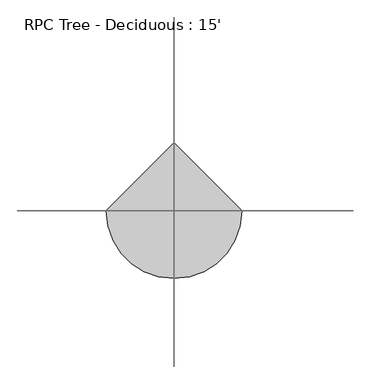
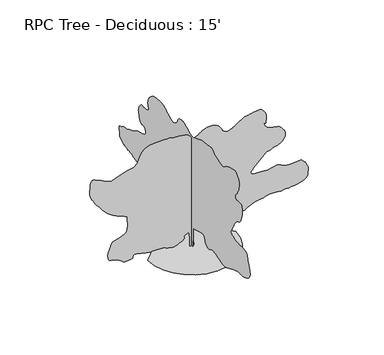
"""IFC4 building model written with IfcOpenShell, lengths in millimetres: geographic element geometry, RPC Tree - Deciduous : 15'."""

from ifc_helpers import new_model, si_unit, origin, place, context, project, spatial, triangles, source, transform, mapped, element, save


def rpc_tree_deciduous_15_10e6bd9b(model_context):
    return source(origin(), model_context, "Body", "Tessellation", [
        triangles([(0.0815727, 123.3442517, 0.0086663), (0.0815727, -127.150442, 0.0086663), (0.0815727, -142.8050915, 829.7731888), (0.0815727, -142.8050915, 1189.8561516), (0.0815727, -455.9234791, 1283.7916969), (0.0815727, -972.5656357, 1456.003569), (0.0815727, -1223.0603748, 1487.3154659), (0.0815727, -1253.1846989, 1460.340659), (0.0815727, -1282.9026524, 1432.5467159), (0.0815727, -1311.7952202, 1403.1018562), (0.0815727, -1339.4557411, 1371.1994431), (0.0815727, -1365.4717403, 1336.0076958), (0.0815727, -1389.4365566, 1296.7076237), (0.0815727, -1410.9313202, 1252.4798), (0.0815727, -1426.1332993, 1206.5185793), (0.0815727, -1434.7564648, 1162.7416729), (0.0815727, -1441.7415035, 1121.4349646), (0.0815727, -1452.0094814, 1082.8650805), (0.0815727, -1470.5006493, 1047.3114367), (0.0815727, -1502.1299686, 1015.040732), (0.0815727, -1551.8378357, 986.3260603), (0.0815727, -1610.353014, 959.8528942), (0.0815727, -1665.3059097, 935.5705101), (0.0815727, -1716.9758663, 915.6696173), (0.0815727, -1765.6294373, 902.34732), (0.0815727, -1811.5462566, 897.781683), (0.0815727, -1855.0056679, 904.1698105), (0.0815727, -1896.2615799, 923.7087341), (0.0815727, -1937.8921783, 949.1722235), (0.0815727, -1981.9865799, 972.178232), (0.0815727, -2028.132019, 993.1332756), (0.0815727, -2075.9221252, 1012.4372572), (0.0815727, -2124.937738, 1030.5156595), (0.0815727, -2174.7852768, 1047.7686035), (0.0815727, -2225.0390408, 1064.6088547), (0.0815727, -2522.4983551, 1017.6378845), (0.0815727, -2603.0164055, 990.8472233), (0.0815727, -2683.5344559, 964.3296558), (0.0815727, -2764.0458206, 938.3582033), (0.0815727, -2844.563871, 913.2058142), (0.0815727, -2925.0819214, 889.1520498), (0.0815727, -3005.5935768, 866.4698587), (0.0815727, -3086.1113365, 845.4259398), (0.0815727, -3169.3661385, 824.8837343), (0.0815727, -3257.5488373, 805.7131021), (0.0815727, -3349.8394249, 791.2033047), (0.0815727, -3445.4196373, 784.6311041), (0.0815727, -3543.4636528, 789.2856165), (0.0815727, -3643.1523354, 808.4562487), (0.0815727, -3743.660154, 845.4259398), (0.0815727, -4495.1442261, 1158.5443274), (0.0815727, -4550.6876381, 1183.5569721), (0.0815727, -4600.2110687, 1205.2802828), (0.0815727, -4649.1886024, 1224.2730915), (0.0815727, -4703.0937424, 1241.0688686), (0.0815727, -4767.4066772, 1256.2199787), (0.0815727, -4847.6070145, 1270.2788589), (0.0815727, -4949.1624435, 1283.7916969), (0.0815727, -5062.9101517, 1293.0563931), (0.0815727, -5174.7335587, 1296.567952), (0.0815727, -5282.7281296, 1298.168145), (0.0815727, -5384.9695633, 1301.6859535), (0.0815727, -5479.5463486, 1310.9506496), (0.0815727, -5564.5347656, 1329.7974644), (0.0815727, -5638.0169083, 1362.068169), (0.0815727, -5707.447554, 1399.0441097), (0.0815727, -5779.3356079, 1431.6323822), (0.0815727, -5850.3987122, 1463.1282795), (0.0815727, -5917.3591599, 1496.8086365), (0.0815727, -5976.9287796, 1535.9754318), (0.0815727, -6025.811261, 1583.8989601), (0.0815727, -6060.7294785, 1643.8746597), (0.0815727, -6088.9364777, 1700.9293167), (0.0815727, -6117.6957687, 1743.7473427), (0.0815727, -6143.7116226, 1781.0790756), (0.0815727, -6163.7011002, 1821.7063923), (0.0815727, -6174.3818436, 1874.3794853), (0.0815727, -6172.4645187, 1947.8680229), (0.0815727, -6154.6650238, 2050.9285927), (0.0815727, -6127.7794556, 2157.8243935), (0.0815727, -6100.6206482, 2242.8190601), (0.0815727, -6072.9153625, 2314.6629307), (0.0815727, -6044.3909409, 2382.1189877), (0.0815727, -6014.7683304, 2453.9630035), (0.0815727, -5983.774292, 2538.9575249), (0.0815727, -5951.1414001, 2645.8533257), (0.0815727, -5922.6995316, 2760.6041702), (0.0815727, -5898.0998703, 2862.2040733), (0.0815727, -5867.7470718, 2949.0214485), (0.0815727, -5822.0585815, 3019.4046524), (0.0815727, -5751.4466125, 3071.7095993), (0.0815727, -5646.3286102, 3104.2977264), (0.0815727, -5497.1167877, 3115.5310524), (0.0815727, -5330.1054703, 3115.7595268), (0.0815727, -5177.0642303, 3117.3533249), (0.0815727, -5036.6146637, 3121.6905602), (0.0815727, -4907.3987137, 3130.1359749), (0.0815727, -4788.0376854, 3144.0551834), (0.0815727, -4677.1668365, 3164.8260086), (0.0815727, -4573.4205528, 3193.8073792), (0.0815727, -4472.8237862, 3223.3858063), (0.0815727, -4376.3293854, 3248.3095757), (0.0815727, -4289.9692497, 3273.4998985), (0.0815727, -4219.7700462, 3303.903566), (0.0815727, -4171.7514656, 3344.435685), (0.0815727, -4151.9456978, 3400.029966), (0.0815727, -4166.3666199, 3475.6140152), (0.0815727, -4193.2524788, 3544.1240776), (0.0815727, -4210.8229179, 3584.7006706), (0.0815727, -4225.1104179, 3611.5865295), (0.0815727, -4242.1349602, 3639.018576), (0.0815727, -4267.922049, 3681.2395454), (0.0815727, -4308.5050369, 3752.4927544), (0.0815727, -4369.8969292, 3867.0151245), (0.0815727, -4431.7393753, 3988.5603218), (0.0815727, -4475.5163544, 4078.342923), (0.0815727, -4509.977623, 4146.764328), (0.0815727, -4543.8865997, 4204.2317505), (0.0815727, -4586.0189117, 4261.1468811), (0.0815727, -4645.1246063, 4327.9233284), (0.0815727, -4729.979892, 4414.969178), (0.0815727, -4825.9661842, 4494.4329323), (0.0815727, -4913.1960342, 4542.680278), (0.0815727, -4992.4760788, 4576.4113586), (0.0815727, -5064.6373718, 4612.3332939), (0.0815727, -5130.5060257, 4667.1529129), (0.0815727, -5190.8942001, 4757.570359), (0.0815727, -5246.6216125, 4900.299147), (0.0815727, -5291.7194412, 5079.6806396), (0.0815727, -5319.8374924, 5261.7985931), (0.0815727, -5331.2484238, 5435.9786591), (0.0815727, -5326.2254745, 5591.5348618), (0.0815727, -5305.0482788, 5717.7852951), (0.0815727, -5267.9830994, 5804.0497971), (0.0815727, -5215.3101517, 5839.6546005), (0.0815727, -5153.0994141, 5844.537442), (0.0815727, -5087.598761, 5846.1379257), (0.0815727, -5019.361647, 5844.9949722), (0.0815727, -4948.9339691, 5841.6608734), (0.0815727, -4876.8616241, 5836.6890839), (0.0815727, -4803.696904, 5830.6185242), (0.0815727, -4729.979892, 5823.9956726), (0.0815727, -4690.177961, 5844.3979156), (0.0815727, -4653.1130722, 5866.4454071), (0.0815727, -4621.5280815, 5891.7816513), (0.0815727, -4598.1600311, 5922.0391068), (0.0815727, -4585.7459633, 5958.8758118), (0.0815727, -4587.0223389, 6003.9224808), (0.0815727, -4604.7323044, 6058.8371521), (0.0815727, -4630.8879753, 6109.0468781), (0.0815727, -4656.7643028, 6144.1877563), (0.0815727, -4684.0184532, 6172.2168594), (0.0815727, -4714.2761993, 6201.0645172), (0.0815727, -4749.1947075, 6238.6755936), (0.0815727, -4790.4125404, 6292.9873947), (0.0815727, -4839.5679703, 6371.9686203), (0.0815727, -4894.9843552, 6476.3622482), (0.0815727, -4949.3025513, 6597.456601), (0.0815727, -4995.6700699, 6728.9654343), (0.0815727, -5027.2611649, 6864.537973), (0.0815727, -5037.2117203, 6997.9513412), (0.0815727, -5018.6762238, 7122.9192947), (0.0815727, -4964.8155579, 7233.0282715), (0.0815727, -4895.8482559, 7332.6593994), (0.0815727, -4832.906749, 7426.2583374), (0.0815727, -4770.5117203, 7507.8562637), (0.0815727, -4703.1890854, 7571.3558762), (0.0815727, -4625.4525513, 7610.7261475), (0.0815727, -4531.8408234, 7619.9970932), (0.0815727, -4416.8615044, 7593.1365234), (0.0815727, -4299.7863831, 7553.8302017), (0.0815727, -4199.1390381, 7526.0167831), (0.0815727, -4108.3530098, 7503.982663), (0.0815727, -4020.8566063, 7481.9479614), (0.0815727, -3930.070578, 7454.1351242), (0.0815727, -3829.423233, 7414.8288025), (0.0815727, -3712.3481117, 7358.2502792), (0.0815727, -3601.2043144, 7291.8927017), (0.0815727, -3515.2569443, 7229.9168335), (0.0815727, -3443.2735474, 7176.7038025), (0.0815727, -3374.0330063, 7136.635318), (0.0815727, -3296.3028671, 7114.0925079), (0.0815727, -3198.8556175, 7113.457663), (0.0815727, -3070.4588036, 7139.111911), (0.0815727, -2923.8500198, 7182.5458878), (0.0815727, -2783.2673218, 7229.8528839), (0.0815727, -2654.7306908, 7277.0970932), (0.0815727, -2544.2726074, 7320.5944382), (0.0815727, -2457.9124718, 7356.345163), (0.0815727, -2401.6769508, 7380.6657715), (0.0815727, -2381.5982346, 7389.5553452), (0.0815727, -2370.504871, 7403.2713684), (0.0815727, -2338.8755516, 7437.8157715), (0.0815727, -2289.1676846, 7483.2182327), (0.0815727, -2223.8516132, 7529.8270157), (0.0815727, -2145.3911407, 7567.6095932), (0.0815727, -2056.2497795, 7586.7863297), (0.0815727, -1958.8853737, 7577.4520157), (0.0815727, -1832.0441334, 7549.956601), (0.0815727, -1666.8552338, 7522.1437637), (0.0815727, -1484.4198578, 7495.7273529), (0.0815727, -1305.8134632, 7472.296225), (0.0815727, -1152.130838, 7453.5636475), (0.0815727, -1044.4539076, 7441.0539459), (0.0815727, -1003.8774599, 7436.5455002), (0.0815727, -988.5866781, 7428.5442444), (0.0815727, -946.7338549, 7407.1449692), (0.0815727, -884.3387535, 7376.1573257), (0.0815727, -807.4276051, 7339.4543335), (0.0815727, -722.0264952, 7300.7828568), (0.0815727, -634.1634716, 7264.0159149), (0.0815727, -549.8589881, 7233.0282715), (0.0815727, -464.0482738, 7201.4685699), (0.0815727, -369.4739594, 7164.7655777), (0.0815727, -268.8747764, 7129.0788025), (0.0815727, -164.9888028, 7100.821225), (0.0815727, -60.5556061, 7086.2796707), (0.0815727, 41.686845, 7091.7403839), (0.0815727, 138.9995371, 7123.4274033), (0.0815727, 241.470726, 7177.021225), (0.0815727, 356.8133586, 7239.6319382), (0.0815727, 478.7282281, 7305.0372482), (0.0815727, 600.9173904, 7366.8224304), (0.0815727, 717.0798494, 7418.7657715), (0.0815727, 820.9213308, 7454.5159149), (0.0815727, 906.138295, 7467.8511475), (0.0815727, 984.8719339, 7467.3430389), (0.0815727, 1070.1840958, 7463.8502289), (0.0815727, 1157.1346024, 7454.3252289), (0.0815727, 1240.8021698, 7435.7199692), (0.0815727, 1316.2465473, 7405.1131165), (0.0815727, 1378.5526279, 7359.3932327), (0.0815727, 1422.7804516, 7295.6389847), (0.0815727, 1452.1745876, 7226.3606552), (0.0815727, 1475.8219814, 7165.019632), (0.0815727, 1497.5453648, 7109.9654343), (0.0815727, 1521.1927586, 7059.609787), (0.0815727, 1550.5868946, 7012.175473), (0.0815727, 1589.5631493, 6966.2009537), (0.0815727, 1641.9632938, 6919.9095932), (0.0815727, 1704.9997078, 6876.0314575), (0.0815727, 1772.4176857, 6839.3284653), (0.0815727, 1842.845509, 6811.0708878), (0.0815727, 1914.9179993, 6792.6557327), (0.0815727, 1987.263438, 6785.4800079), (0.0815727, 2058.5103973, 6790.9413025), (0.0815727, 2127.2999485, 6810.308725), (0.0815727, 2197.5881001, 6840.344101), (0.0815727, 2273.6292435, 6876.158194), (0.0815727, 2354.4647163, 6916.734787), (0.0815727, 2439.1357109, 6961.1210312), (0.0815727, 2526.6829834, 7008.4286087), (0.0815727, 2616.1417671, 7057.6413025), (0.0815727, 2706.5658989, 7107.8062637), (0.0815727, 2764.1222694, 7147.7474304), (0.0815727, 2824.828157, 7186.1014847), (0.0815727, 2891.8333694, 7221.1534149), (0.0815727, 2968.287133, 7251.3161087), (0.0815727, 3057.3395462, 7274.8111862), (0.0815727, 3162.140126, 7290.1782715), (0.0815727, 3285.8317039, 7295.6389847), (0.0815727, 3428.1985954, 7292.5909149), (0.0815727, 3581.2398354, 7282.6851242), (0.0815727, 3736.4719299, 7264.8414459), (0.0815727, 3885.4110947, 7237.9808762), (0.0815727, 4019.5610458, 7200.9604614), (0.0815727, 4130.4257904, 7152.7006165), (0.0815727, 4209.5276482, 7092.121756), (0.0815727, 4267.1793617, 7032.8125854), (0.0815727, 4319.8967834, 6985.5050079), (0.0815727, 4368.5060257, 6945.0557327), (0.0815727, 4413.8323288, 6906.2575195), (0.0815727, 4456.6884338, 6863.9025467), (0.0815727, 4497.9062668, 6812.785318), (0.0815727, 4538.3049637, 6747.6980118), (0.0815727, 4572.9949974, 6674.7995544), (0.0815727, 4597.2775269, 6603.5527405), (0.0815727, 4612.2443459, 6533.639566), (0.0815727, 4619.0009102, 6464.8687637), (0.0815727, 4618.6390137, 6396.9240738), (0.0815727, 4612.2443459, 6329.5060959), (0.0815727, 4600.9287575, 6262.3613571), (0.0815727, 4582.7615524, 6201.5662308), (0.0815727, 4559.1202629, 6151.718692), (0.0815727, 4536.0190567, 6110.3677277), (0.0815727, 4519.4965187, 6075.0361633), (0.0815727, 4515.572049, 6043.2735672), (0.0815727, 4530.2723145, 6012.5969513), (0.0815727, 4569.6170059, 5980.5547211), (0.0815727, 4622.5187187, 5951.4780075), (0.0815727, 4674.5951912, 5930.0723373), (0.0815727, 4726.9507164, 5914.419223), (0.0815727, 4780.6718559, 5902.5955261), (0.0815727, 4836.8629028, 5892.6897354), (0.0815727, 4896.6098373, 5882.7839447), (0.0815727, 4961.0117203, 5870.9660614), (0.0815727, 5027.1530319, 5867.5435959), (0.0815727, 5091.3706238, 5878.0848129), (0.0815727, 5153.6767044, 5893.5594498), (0.0815727, 5214.0654602, 5904.9261978), (0.0815727, 5272.5299149, 5903.1420044), (0.0815727, 5329.0828583, 5879.1830017), (0.0815727, 5383.7184769, 5823.9956726), (0.0815727, 5436.1693451, 5753.612178), (0.0815727, 5485.0518265, 5688.4359238), (0.0815727, 5528.7334625, 5625.9961304), (0.0815727, 5565.5695862, 5563.8295761), (0.0815727, 5593.9097168, 5499.4660629), (0.0815727, 5612.1213959, 5430.4545776), (0.0815727, 5618.5605377, 5354.3179459), (0.0815727, 5610.8005463, 5269.2405807), (0.0815727, 5589.0710587, 5175.9462753), (0.0815727, 5555.7079788, 5075.8006439), (0.0815727, 5513.0297699, 4970.180928), (0.0815727, 5463.3665222, 4860.4530327), (0.0815727, 5409.0547211, 4747.9883858), (0.0815727, 5352.4064346, 4634.1520203), (0.0815727, 5252.4003296, 4646.6995102), (0.0815727, 5156.2294556, 4654.0528404), (0.0815727, 5067.7296249, 4650.9922714), (0.0815727, 4990.7232788, 4632.3230621), (0.0815727, 4929.0584381, 4592.8452393), (0.0815727, 4886.5645203, 4527.3448769), (0.0815727, 4867.0761749, 4430.621711), (0.0815727, 4871.5020676, 4330.9394234), (0.0815727, 4896.7435501, 4256.1748009), (0.0815727, 4940.6088959, 4200.5805199), (0.0815727, 5000.9023087, 4158.4037338), (0.0815727, 5075.4384567, 4123.8979912), (0.0815727, 5162.0273575, 4091.3034691), (0.0815727, 5258.4708893, 4054.8798203), (0.0815727, 5351.5872986, 4023.7965431), (0.0815727, 5434.0229645, 4005.584864), (0.0815727, 5512.3437653, 3992.033947), (0.0815727, 5593.1347641, 3974.9143524), (0.0815727, 5682.9618393, 3946.0216393), (0.0815727, 5788.3972641, 3897.1394485), (0.0815727, 5916.0197067, 3820.0441544), (0.0815727, 6053.0462265, 3736.7893524), (0.0815727, 6182.1290451, 3671.6130981), (0.0815727, 6302.9885284, 3619.5747047), (0.0815727, 6415.3386475, 3575.7596466), (0.0815727, 6518.970694, 3535.2278183), (0.0815727, 6613.5224808, 3493.0510323), (0.0815727, 6698.8027405, 3444.3022636), (0.0815727, 6781.9877792, 3403.4527222), (0.0815727, 6869.5545273, 3382.0467613), (0.0815727, 6960.1053955, 3370.769252), (0.0815727, 7052.3073257, 3360.316983), (0.0815727, 7144.7633102, 3341.375116), (0.0815727, 7236.1397095, 3304.6340446), (0.0815727, 7325.0395157, 3240.7783493), (0.0815727, 7409.7482986, 3183.0376877), (0.0815727, 7487.0912521, 3158.4316315), (0.0815727, 7553.4488297, 3148.347654), (0.0815727, 7605.3282211, 3134.149102), (0.0815727, 7639.1104614, 3097.2240303), (0.0815727, 7651.2387909, 3018.9474129), (0.0815727, 7638.158194, 2880.6889915), (0.0815727, 7621.9655777, 2732.0736443), (0.0815727, 7619.7430389, 2627.2733551), (0.0815727, 7620.5052017, 2554.5214005), (0.0815727, 7613.3294769, 2502.0260582), (0.0815727, 7587.2944382, 2458.0269997), (0.0815727, 7531.3507599, 2410.7384617), (0.0815727, 7434.6403839, 2348.3941566), (0.0815727, 7333.6122482, 2287.8215458), (0.0815727, 7262.6828568, 2249.1627136), (0.0815727, 7207.882132, 2225.5661888), (0.0815727, 7155.3039459, 2210.180064), (0.0815727, 7090.9154343, 2196.1656578), (0.0815727, 7000.8720932, 2176.6774578), (0.0815727, 6871.0149033, 2144.8639927), (0.0815727, 6728.3305893, 2114.0538094), (0.0815727, 6605.2671707, 2097.7597458), (0.0815727, 6496.809256, 2089.4095287), (0.0815727, 6397.622287, 2082.42449), (0.0815727, 6302.5309982, 2070.2388966), (0.0815727, 6206.3607056, 2046.2739349), (0.0815727, 6103.8907974, 2003.9640175), (0.0815727, 5978.6432098, 1954.9420097), (0.0815727, 5826.5606323, 1914.6829845), (0.0815727, 5661.0544556, 1882.3678059), (0.0815727, 5495.5482788, 1857.171088), (0.0815727, 5343.4657013, 1838.2734043), (0.0815727, 5218.2181137, 1824.8559093), (0.0815727, 5133.230278, 1816.0929268), (0.0815727, 5074.4861893, 1810.7970291), (0.0815727, 5017.9332458, 1806.3202675), (0.0815727, 4961.9261993, 1799.6591915), (0.0815727, 4904.8267776, 1787.7910206), (0.0815727, 4844.9845001, 1767.7059093), (0.0815727, 4780.7669083, 1736.3941578), (0.0815727, 4710.5171265, 1690.8456299), (0.0815727, 4645.1565811, 1642.0965706), (0.0815727, 4592.1214462, 1599.9199299), (0.0815727, 4544.5534195, 1559.3879562), (0.0815727, 4495.6267548, 1515.5728981), (0.0815727, 4438.4767548, 1463.53465), (0.0815727, 4366.2709877, 1398.3583958), (0.0815727, 4272.1511513, 1315.1035938), (0.0815727, 4191.2714951, 1234.3569237), (0.0815727, 4150.3774796, 1175.2511564), (0.0815727, 4130.0194199, 1130.655114), (0.0815727, 4110.7534447, 1093.4568758), (0.0815727, 4073.1487633, 1056.5316587), (0.0815727, 3997.7426102, 1012.7547523), (0.0815727, 3865.097509, 955.0205584), (0.0815727, 3713.376828, 898.5564177), (0.0815727, 3588.770771, 859.8975855), (0.0815727, 3483.8815338, 833.8308626), (0.0815727, 3391.3177071, 815.1618713), (0.0815727, 3303.6814865, 798.6899843), (0.0815727, 3213.5811722, 779.195462), (0.0815727, 3113.6195412, 751.4904671), (0.0815727, 3025.6595032, 724.972827), (0.0815727, 2965.912278, 709.955139), (0.0815727, 2918.4904633, 702.6082037), (0.0815727, 2867.506366, 699.0902498), (0.0815727, 2797.078688, 695.5786909), (0.0815727, 2691.3194458, 688.2317556), (0.0815727, 2534.3473412, 673.213995), (0.0815727, 2373.6353485, 655.8213793), (0.0815727, 2257.0177574, 643.3626921), (0.0815727, 2169.1527718, 635.0060801), (0.0815727, 2094.7054264, 629.9413456), (0.0815727, 2018.3467152, 627.3397602), (0.0815727, 1924.7287376, 626.3808798), (0.0815727, 1798.5224876, 626.2437515), (0.0815727, 1676.8374733, 627.2025593), (0.0815727, 1595.6845779, 630.0778925), (0.0815727, 1538.0773384, 634.8714952), (0.0815727, 1487.0487671, 641.5783533), (0.0815727, 1425.6125462, 650.2079865), (0.0815727, 1336.7887527, 660.7489855), (0.0815727, 1203.5975367, 673.213995), (0.0815727, 1055.4839029, 688.3207037), (0.0815727, 931.1954138, 705.8911428), (0.0815727, 827.7221512, 724.5601341), (0.0815727, 742.0480202, 742.9560316), (0.0815727, 671.1629574, 759.7073347), (0.0815727, 612.0546467, 773.4487198), (0.0815727, 561.7093549, 782.8022913), (0.0815727, 512.9153129, 792.7083), (0.0815727, 460.8358246, 808.361051), (0.0815727, 406.0169323, 828.814381), (0.0815727, 349.0079121, 853.0967651), (0.0815727, 290.354897, 880.2557178), (0.0815727, 230.6071449, 909.3259638), (0.0815727, 170.3113704, 939.3614851), (0.0815727, 76.3764972, 798.4613646), (114.7946192, 0.0003886, 0.0), (-120.0435266, 0.0003886, 0.0), (-120.0435266, 0.0003532, 579.2677308), (-167.011917, 0.0003297, 939.3550901), (-480.1290147, 0.0003415, 767.1368231), (-467.5769829, 0.0003415, 726.7889952), (-460.2281219, 0.0003532, 685.8886574), (-463.2862927, 0.0003532, 643.902412), (-481.95463, 0.0003532, 600.2639783), (-521.4370311, 0.0003532, 554.4373424), (-586.9359764, 0.0003532, 505.8719201), (-683.6534014, 0.000365, 454.0203612), (-780.0082758, 0.000365, 409.28908), (-846.7848684, 0.000365, 379.8943262), (-892.7524841, 0.000365, 362.0025767), (-926.6614609, 0.000365, 351.7778011), (-957.2938934, 0.000365, 345.3884382), (-993.3935795, 0.000365, 338.9978036), (-1043.7427591, 0.000365, 328.7736457), (-1099.9274837, 0.000365, 319.8728808), (-1150.0925177, 0.000365, 318.9140004), (-1197.7873535, 0.000365, 324.2549898), (-1246.5807415, 0.000365, 334.250528), (-1300.0286419, 0.000365, 347.259763), (-1361.6998775, 0.000365, 361.6374464), (-1435.1375462, 0.000365, 375.7407643), (-1501.2282795, 0.000365, 390.8493261), (-1545.9640663, 0.000365, 408.4223087), (-1580.558757, 0.000365, 427.0913), (-1616.2522179, 0.000365, 445.4853444), (-1664.2707985, 0.000365, 462.2366475), (-1735.8417206, 0.000365, 475.9754891), (-1842.1914791, 0.000365, 485.3322218), (-1948.0839981, 0.000365, 491.0833969), (-2020.2961601, 0.000365, 494.9168839), (-2073.0582012, 0.000365, 496.8352261), (-2120.6196877, 0.000365, 496.8339543), (-2177.2172504, 0.000365, 494.9175379), (-2257.0939156, 0.000365, 491.0833969), (-2374.492709, 0.000365, 485.3322218), (-2504.6674667, 0.000365, 484.8299269), (-2616.4972687, 0.000365, 494.7346639), (-2714.6302322, 0.0003532, 512.034589), (-2803.7271194, 0.0003532, 533.7147337), (-2888.4422974, 0.0003532, 556.7652526), (-2973.4307144, 0.0003532, 578.1723398), (-3063.3531326, 0.0003532, 594.9236429), (-3155.1422974, 0.0003532, 612.2680058), (-3241.7245125, 0.0003532, 633.9945139), (-3321.7408493, 0.0003532, 654.9006506), (-3393.8131943, 0.0003532, 669.7786669), (-3456.5704102, 0.0003532, 673.4298975), (-3508.6529869, 0.0003532, 660.6537151), (-3548.6833923, 0.0003532, 626.2348131), (-3571.6386772, 0.0003532, 581.2298567), (-3580.903228, 0.0003532, 540.3327164), (-3587.7039757, 0.0003532, 503.8183391), (-3603.2678513, 0.000365, 471.9584742), (-3638.82789, 0.000365, 445.0294129), (-3705.604628, 0.000365, 423.3022508), (-3814.8308098, 0.000365, 407.0532426), (-3930.4007904, 0.000365, 395.8696229), (-4014.7540718, 0.000365, 390.4378324), (-4076.9206261, 0.000365, 392.6755955), (-4125.9426338, 0.000365, 404.4967489), (-4170.8561714, 0.000365, 427.8209066), (-4220.6973152, 0.000365, 464.5645577), (-4284.5082458, 0.0003532, 516.644046), (-4354.0726044, 0.0003532, 570.7314059), (-4417.3312431, 0.0003532, 613.865074), (-4477.5801819, 0.0003532, 648.5125231), (-4538.1081734, 0.0003532, 677.1256021), (-4602.1923431, 0.0003415, 702.1890432), (-4673.1220253, 0.0003415, 726.1476099), (-4754.1859726, 0.0003415, 751.4840721), (-4836.5262955, 0.0003415, 772.7946899), (-4908.7387482, 0.0003415, 787.8124506), (-4970.2634811, 0.0003415, 803.6556696), (-5020.5621552, 0.0003415, 827.4364128), (-5059.0877106, 0.0003415, 866.279318), (-5085.2872742, 0.0003297, 927.3028461), (-5098.6161118, 0.0003297, 1017.6315622), (-5104.0454315, 0.0003179, 1116.1326719), (-5105.6453339, 0.0003179, 1199.8447134), (-5101.4926804, 0.0003179, 1273.1490326), (-5089.6689835, 0.0003061, 1340.4273388), (-5068.2633133, 0.0003061, 1406.0608326), (-5035.3513687, 0.0003061, 1474.4376183), (-4989.0216385, 0.0002944, 1549.9327194), (-4951.962854, 0.0002944, 1625.1103981), (-4937.9038284, 0.0002826, 1691.2456055), (-4931.5094513, 0.0002826, 1750.8085396), (-4917.4510071, 0.0002826, 1806.2695438), (-4880.3922226, 0.0002826, 1860.0857357), (-4804.9860695, 0.0002708, 1914.7210636), (-4675.9032509, 0.0002708, 1972.639476), (-4515.9659203, 0.0002708, 2026.5889446), (-4362.6069672, 0.0002708, 2072.601107), (-4222.3864563, 0.000259, 2118.0606869), (-4101.8888695, 0.000259, 2170.3720287), (-4007.6803757, 0.000259, 2236.9200016), (-3946.3329575, 0.0002473, 2325.1024097), (-3924.4255737, 0.0002473, 2442.3169121), (-3920.3171036, 0.0002355, 2554.6929016), (-3910.7284447, 0.0002355, 2632.0166702), (-3899.7747528, 0.0002237, 2687.1537117), (-3891.5578125, 0.0002237, 2732.9753334), (-3890.1924889, 0.0002237, 2782.3656326), (-3899.7747528, 0.0002237, 2848.1834175), (-3924.4255737, 0.0002119, 2943.3063904), (-3942.1800133, 0.0002119, 3041.3948799), (-3938.0270691, 0.0002002, 3112.6480888), (-3926.4766113, 0.0002002, 3164.7245613), (-3922.050428, 0.0002002, 3205.3008636), (-3939.2589706, 0.0002002, 3242.0483299), (-3992.6118187, 0.0001884, 3282.6249229), (-4096.6374458, 0.0001884, 3334.7011047), (-4224.5770203, 0.0001884, 3390.7970993), (-4341.836142, 0.0001884, 3440.3205299), (-4451.1512718, 0.0001766, 3486.2883636), (-4555.265847, 0.0001766, 3531.7036148), (-4656.9166191, 0.0001766, 3579.5823784), (-4758.8406303, 0.0001766, 3632.9416214), (-4863.7743416, 0.0001648, 3694.7904625), (-4965.1074005, 0.0001648, 3760.6971954), (-5057.1250397, 0.0001648, 3827.1562202), (-5143.9424149, 0.0001531, 3898.5428513), (-5229.6610199, 0.0001531, 3979.2385071), (-5318.389325, 0.0001413, 4073.631292), (-5414.2427765, 0.0001413, 4186.1023338), (-5521.3228683, 0.0001295, 4321.0208427), (-5618.6808792, 0.0001295, 4440.9786369), (-5688.6580032, 0.0001177, 4517.6547707), (-5740.2769455, 0.0001177, 4569.1469765), (-5782.5871536, 0.0001177, 4613.5082222), (-5824.6241226, 0.000106, 4668.8292641), (-5875.4303238, 0.000106, 4753.1825455), (-5944.0296249, 9.42e-05, 4884.6338242), (-6018.7500641, 9.42e-05, 5015.1328354), (-6081.6973846, 8.24e-05, 5100.4386749), (-6132.5861389, 8.24e-05, 5164.3894226), (-6171.1558777, 8.24e-05, 5230.7975784), (-6197.1275482, 7.06e-05, 5323.5012222), (-6210.2279114, 5.89e-05, 5466.319249), (-6210.1831467, 4.71e-05, 5683.0827621), (-6198.6326889, 3.53e-05, 5915.7784424), (-6177.2270187, 2.35e-05, 6093.4257385), (-6145.6865021, 2.35e-05, 6220.4069412), (-6103.7384811, 1.18e-05, 6301.102597), (-6051.1155304, 1.18e-05, 6339.9008102), (-5987.5333649, 1.18e-05, 6341.1774765), (-5912.7239777, 1.18e-05, 6309.3195374), (-5832.2945847, 1.18e-05, 6266.6919067), (-5752.4180649, 1.18e-05, 6230.9033936), (-5673.6403152, 2.35e-05, 6199.2297455), (-5596.5002563, 2.35e-05, 6168.9211304), (-5521.5513428, 2.35e-05, 6137.240506), (-5449.345285, 2.35e-05, 6101.4583878), (-5380.4227478, 2.35e-05, 6058.8249435), (-5313.7797226, 3.53e-05, 6016.4257874), (-5247.961647, 3.53e-05, 5982.2371765), (-5182.8295761, 3.53e-05, 5954.8940781), (-5118.2439835, 3.53e-05, 5933.031459), (-5054.0647614, 3.53e-05, 5915.2767288), (-4990.164592, 3.53e-05, 5900.2590408), (-4926.403949, 3.53e-05, 5886.6127808), (-4206.2255241, 2.35e-05, 6137.1073746), (-4081.6197578, 2.35e-05, 6173.0737839), (-3953.1781792, 2.35e-05, 6202.4679199), (-3826.6545067, 1.18e-05, 6228.2994827), (-3707.795192, 1.18e-05, 6253.5915436), (-3602.3597672, 1.18e-05, 6281.3410126), (-3516.0952652, 1.18e-05, 6314.570961), (-3454.747847, 1.18e-05, 6356.2841125), (-3408.8311729, 1.18e-05, 6405.1788025), (-3365.3780113, 0.0, 6457.883725), (-3324.9348404, 0.0, 6514.4622482), (-3288.053952, 0.0, 6574.851004), (-3255.2818245, -1.18e-05, 6639.049411), (-3227.1701683, -1.18e-05, 6707.1214188), (-3204.2532532, -1.18e-05, 6779.0030777), (-3180.5169113, -2.35e-05, 6851.6474808), (-3150.4812447, -2.35e-05, 6920.9258102), (-3115.5182625, -2.35e-05, 6985.6323257), (-3076.999102, -3.53e-05, 7044.3060699), (-3036.2829826, -3.53e-05, 7095.5506165), (-2994.7477272, -3.53e-05, 7138.0323257), (-2953.7583687, -3.53e-05, 7170.4169769), (-2909.2131226, -3.53e-05, 7203.119632), (-2854.2539772, -4.71e-05, 7244.3310699), (-2786.1566803, -4.71e-05, 7289.0986862), (-2702.1716904, -4.71e-05, 7332.532663), (-2599.5619652, -4.71e-05, 7369.6164459), (-2475.5910439, -4.71e-05, 7395.5247482), (-2327.5217388, -4.71e-05, 7405.2398529), (-2160.1929989, -4.71e-05, 7408.5419769), (-1985.7394032, -5.89e-05, 7416.1618607), (-1812.3845776, -5.89e-05, 7424.9252792), (-1648.3386314, -5.89e-05, 7431.5289459), (-1501.8251907, -5.89e-05, 7432.6085312), (-1381.0482605, -5.89e-05, 7424.9252792), (-1294.2374256, -4.71e-05, 7405.2398529), (-1221.7521698, -4.71e-05, 7382.8243607), (-1139.9578892, -4.71e-05, 7367.7752792), (-1051.0452204, -4.71e-05, 7357.996225), (-957.1986231, -4.71e-05, 7351.2012909), (-860.6151289, -4.71e-05, 7345.2324692), (-763.4855925, -4.71e-05, 7337.8666397), (-668.0006504, -4.71e-05, 7326.944632), (-573.5616111, -4.71e-05, 7314.0541397), (-479.9461407, -4.71e-05, 7300.6555389), (-389.890482, -4.71e-05, 7284.2088684), (-306.1340029, -4.71e-05, 7262.3014847), (-231.4148536, -4.71e-05, 7232.4567947), (-168.4717843, -3.53e-05, 7192.1976242), (-120.0435266, -3.53e-05, 7139.111911), (-80.0594937, -3.53e-05, 7080.8189575), (-41.7188471, -3.53e-05, 7027.7960312), (-6.6642587, -2.35e-05, 6981.3139847), (23.4606365, -2.35e-05, 6942.833194), (47.0129053, -2.35e-05, 6913.623349), (62.3492284, -2.35e-05, 6895.0814575), (67.8262288, -2.35e-05, 6888.6045273), (83.7107425, -2.35e-05, 6894.0018723), (125.885521, -2.35e-05, 6909.0509537), (186.1362039, -2.35e-05, 6931.7205002), (256.2452602, -2.35e-05, 6960.1687637), (327.9976756, -2.35e-05, 6992.4266785), (393.1772364, -3.53e-05, 7026.5897095), (443.5682739, -3.53e-05, 7060.8161087), (496.8803178, -3.53e-05, 7100.18638), (571.0063891, -3.53e-05, 7147.81138), (658.0057663, -3.53e-05, 7198.4205002), (749.9283531, -4.71e-05, 7246.8710312), (838.8473442, -4.71e-05, 7287.8923645), (916.8062485, -4.71e-05, 7316.3400467), (975.8676144, -4.71e-05, 7326.944632), (1351.6096504, -4.71e-05, 7311.3234924), (1418.4307171, -4.71e-05, 7277.7319382), (1483.6133663, -4.71e-05, 7243.8229614), (1545.5068268, -3.53e-05, 7209.4058762), (1602.4662861, -3.53e-05, 7174.1638412), (1652.8598671, -3.53e-05, 7137.8416397), (1695.0365078, -3.53e-05, 7100.1224304), (1727.3516865, -3.53e-05, 7060.8161087), (1753.2787376, -3.53e-05, 7020.1127792), (1777.5611217, -2.35e-05, 6978.5839188), (1800.4719326, -2.35e-05, 6936.3562637), (1822.2905136, -2.35e-05, 6893.557132), (1843.2835636, -2.35e-05, 6850.3772095), (1863.7369663, -1.18e-05, 6806.9432327), (1883.9108803, -1.18e-05, 6763.3185699), (1927.4973186, -1.18e-05, 6733.3465622), (1970.9503349, -1.18e-05, 6704.5814575), (2014.1302574, -1.18e-05, 6678.2923645), (2056.8975597, -1.18e-05, 6655.6861862), (2099.1186745, -1.18e-05, 6638.033194), (2140.6539299, -1.18e-05, 6626.5397095), (2181.3701946, 0.0, 6622.4126358), (2225.3692532, -1.18e-05, 6626.2856552), (2276.4931675, -1.18e-05, 6637.7791397), (2334.1892097, -1.18e-05, 6656.9564575), (2397.905088, -1.18e-05, 6683.7530777), (2467.1011551, -1.18e-05, 6718.2974808), (2541.2309326, -1.18e-05, 6760.4611862), (2619.7360245, -1.18e-05, 6810.308725), (2709.702626, -2.35e-05, 6871.4590622), (2814.1790977, -2.35e-05, 6943.02388), (2926.5995613, -3.53e-05, 7018.1442947), (3040.3914528, -3.53e-05, 7090.0259537), (3148.9763947, -3.53e-05, 7151.748349), (3245.7885086, -3.53e-05, 7196.4520157), (3324.2491264, -4.71e-05, 7217.3437637), (3393.6291939, -4.71e-05, 7225.471756), (3467.1177315, -4.71e-05, 7236.0123917), (3544.0287346, -4.71e-05, 7248.5854614), (3623.6767799, -4.71e-05, 7262.8095932), (3705.3758629, -4.71e-05, 7278.3034149), (3788.4466644, -4.71e-05, 7294.5593994), (3872.2092842, -4.71e-05, 7311.3234924), (3949.069709, -4.71e-05, 7321.0391785), (4024.1584396, -4.71e-05, 7328.6590622), (4095.6784927, -4.71e-05, 7332.2786087), (4161.8645691, -4.71e-05, 7329.6752792), (4220.9257896, -4.71e-05, 7318.8166397), (4271.0907509, -4.71e-05, 7297.734787), (4310.5688644, -4.71e-05, 7264.3333374), (4349.0941292, -4.71e-05, 7218.6134537), (4394.4649063, -3.53e-05, 7162.9877792), (4442.0265381, -3.53e-05, 7099.170163), (4487.1240761, -3.53e-05, 7028.8122482), (4525.097049, -2.35e-05, 6953.5011475), (4551.2971939, -2.35e-05, 6874.888504), (4561.0634583, -1.18e-05, 6794.6242172), (4559.6981346, -1.18e-05, 6717.7893723), (4555.8629036, -1.18e-05, 6647.4948257), (4549.9699493, 0.0, 6582.6615738), (4542.4390137, 0.0, 6522.272818), (4533.6758858, 0.0, 6465.122818), (4524.0939125, 1.18e-05, 6410.1319885), (4514.0988831, 1.18e-05, 6356.2841125), (4481.0535164, 1.18e-05, 6369.047287), (4451.0181404, 1.18e-05, 6378.0008102), (4427.0085594, 1.18e-05, 6379.2710815), (4412.0353455, 1.18e-05, 6369.047287), (4409.1143028, 1.18e-05, 6343.5075668), (4421.2557129, 1.18e-05, 6298.7783203), (4451.4750893, 1.18e-05, 6231.0429199), (4494.0582458, 2.35e-05, 6158.0119125), (4539.1116005, 2.35e-05, 6099.2236404), (4583.3391335, 2.35e-05, 6053.5793335), (4623.4584869, 3.53e-05, 6019.9819656), (4656.1864311, 3.53e-05, 5997.3438126), (4678.2336319, 3.53e-05, 5984.5614532), (4686.3107552, 3.53e-05, 5980.5483261), (5015.0880707, 3.53e-05, 5902.2653137), (5265.5832458, 3.53e-05, 5855.3007385), (5390.8302521, 4.71e-05, 5792.6772354), (5460.8009811, 4.71e-05, 5712.3879501), (5527.8951416, 5.89e-05, 5633.4700928), (5589.2425598, 5.89e-05, 5557.2892776), (5641.9602722, 5.89e-05, 5485.2169327), (5683.1781052, 7.06e-05, 5418.6244858), (5710.0130951, 7.06e-05, 5358.8769699), (5719.6014633, 7.06e-05, 5307.3469757), (5718.8712753, 7.06e-05, 5253.2130707), (5713.7593781, 8.24e-05, 5186.7543365), (5699.8846436, 8.24e-05, 5110.9857056), (5672.8653625, 9.42e-05, 5028.9186218), (5628.3140121, 9.42e-05, 4943.562204), (5561.8546967, 9.42e-05, 4857.9322563), (5469.1068695, 0.000106, 4775.0457458), (5371.2913284, 0.000106, 4711.1391815), (5288.5382401, 0.000106, 4674.0806877), (5214.821228, 0.000106, 4654.2688156), (5144.120311, 0.0001177, 4642.1274055), (5070.403299, 0.0001177, 4628.0686707), (4987.6560242, 0.0001177, 4602.5097656), (4889.8410645, 0.0001177, 4555.8629036), (4798.1405571, 0.0001177, 4512.5431641), (4731.3641098, 0.0001177, 4494.9727249), (4679.922773, 0.0001177, 4490.5468323), (4634.2345734, 0.0001177, 4486.6668365), (4584.7108521, 0.0001177, 4470.7346695), (4521.7632408, 0.0001295, 4430.1583672), (4435.8161613, 0.0001295, 4352.3325943), (3762.6148109, 0.0001648, 3710.4432861), (3713.1800377, 0.0001766, 3640.3330307), (3669.0920311, 0.0001766, 3572.2799171), (3635.678373, 0.0001766, 3508.3355644), (3618.2919342, 0.0001884, 3450.5440338), (3622.260878, 0.0001884, 3400.9761292), (3652.9313896, 0.0001884, 3361.6759117), (3715.6502357, 0.0001884, 3334.7011047), (3797.3493187, 0.0001884, 3319.7342857), (3882.3377357, 0.0001884, 3312.7047729), (3971.9869148, 0.0001884, 3310.0569695), (4067.6560753, 0.0001884, 3308.2280113), (4170.7163544, 0.0001884, 3303.6623016), (4282.5461563, 0.0001884, 3292.8039528), (4404.5044098, 0.0001884, 3272.0776016), (4543.1755966, 0.0001884, 3266.3753334), (4699.0934052, 0.0001884, 3291.6165253), (4864.5995819, 0.0001884, 3330.8213997), (5032.0172699, 0.0001884, 3367.0162834), (5193.6882156, 0.0001884, 3383.2213989), (5341.9419571, 0.0001884, 3362.4569687), (5469.1068695, 0.0001884, 3287.7365295), (5617.4489777, 0.0002002, 3209.2759117), (5818.1024277, 0.0002002, 3177.6403427), (6046.6832428, 0.0002002, 3176.4084412), (6278.8266312, 0.0002002, 3189.1466171), (6490.1416397, 0.0002002, 3199.414595), (6656.3216125, 0.0002002, 3190.7848892), (6752.9046707, 0.0002002, 3146.830014), (6802.8795273, 0.0002002, 3088.4545074), (6845.9955002, 0.0002119, 3044.0426834), (6883.0798645, 0.0002119, 3008.3939873), (6915.0203568, 0.0002119, 2976.307283), (6942.5157715, 0.0002119, 2942.5762024), (6966.5189575, 0.0002119, 2901.9996094), (6987.7275467, 0.0002237, 2849.370845), (7010.2064072, 0.0002237, 2796.2848412), (7035.4798645, 0.0002237, 2752.514257), (7060.435318, 0.0002237, 2710.1089966), (7082.0886475, 0.0002355, 2661.1314629), (7097.519101, 0.0002355, 2597.6443497), (7103.5518723, 0.0002355, 2511.6969795), (7097.3284149, 0.0002473, 2395.3523369), (7089.3911087, 0.000259, 2272.8419369), (7083.9937637, 0.000259, 2170.6006485), (7068.1819382, 0.000259, 2083.9675644), (7029.0029343, 0.0002708, 2008.2883175), (6953.7552017, 0.0002708, 1938.90825), (6829.4860428, 0.0002826, 1871.1728497), (6643.3038025, 0.0002826, 1800.4274586), (6436.1036591, 0.0002826, 1739.9945194), (6252.6776459, 0.0002826, 1702.2946404), (6086.2564087, 0.0002944, 1681.2951954), (5929.9769943, 0.0002944, 1670.9827435), (5776.9735428, 0.0002944, 1665.3185543), (5620.4144943, 0.0002944, 1658.2891869), (5453.4479416, 0.0002944, 1643.8682648), (5297.9423172, 0.0002944, 1636.4261318), (5171.7366486, 0.0002944, 1647.6084435), (5061.9578842, 0.0002944, 1667.2807892), (4955.7475067, 0.0002826, 1685.3147175), (4840.2220001, 0.0002826, 1691.5631733), (4702.5161613, 0.0002944, 1675.9103497), (4529.7517067, 0.0002944, 1628.2091915), (4358.2700226, 0.0002944, 1575.9487186), (4225.6757904, 0.0002944, 1547.5133904), (4121.0086327, 0.0002944, 1534.1403694), (4033.3279381, 0.0002944, 1527.0663826), (3951.6733292, 0.0002944, 1517.5223431), (3865.0847191, 0.0002944, 1496.7579128), (3762.6148109, 0.0003061, 1455.9973194), (3666.1265144, 0.0003061, 1411.0393078), (3598.391114, 0.0003061, 1380.0449787), (3549.8199509, 0.0003061, 1357.8200272), (3510.8438416, 0.0003061, 1339.1509632), (3471.8610466, 0.0003061, 1318.8373775), (3423.2962784, 0.0003061, 1291.6784248), (3355.560878, 0.0003179, 1252.4735504), (3289.4701447, 0.0003179, 1213.4019527), (3244.7406075, 0.0003179, 1187.2018805), (3210.1395218, 0.0003179, 1169.4916969), (3174.4463516, 0.0003179, 1155.8900562), (3126.4274803, 0.0003179, 1142.0153217), (3054.8568489, 0.0003179, 1123.4796799), (2948.506945, 0.0003179, 1095.9142839), (2275.30574, 0.0003297, 970.666987), (2133.9928539, 0.0003297, 936.7071413), (2022.8044373, 0.0003297, 913.7011328), (1927.7702671, 0.0003297, 899.185013), (1834.9333466, 0.0003415, 890.6951242), (1730.3172031, 0.0003415, 885.767518), (1599.958009, 0.0003415, 881.932069), (1429.8861225, 0.0003415, 876.7314417), (1241.4689896, 0.0003415, 871.8419872), (1067.0217888, 0.0003415, 870.2481165), (909.0021463, 0.0003415, 871.39107), (769.87372, 0.0003415, 874.7184832), (652.1129574, 0.0003415, 879.6968857), (558.1793741, 0.0003415, 885.767518), (490.5347749, 0.0003415, 892.3841927), (438.2272845, 0.0003297, 903.2046078), (388.3842513, 0.0003297, 921.4163595), (340.5947991, 0.0003297, 945.7876917), (294.4487423, 0.0003297, 975.0928797), (249.5352229, 0.0003297, 1008.093845), (205.4427289, 0.0003297, 1043.5586134), (161.7617469, 0.0003297, 1080.2552107), (99.1380621, 0.0003179, 1283.7790524), (67.8262288, 0.0003415, 735.8249989), (-2686.671183, 0.0, 0.0079127), (-2615.6400536, -615.6068281, 0.0079127), (-2413.360976, -1180.9407801, 0.0079127), (-2096.0134861, -1679.8156345, 0.0079127), (-1679.8156345, -2096.0198811, 0.0079127), (-1180.9407801, -2413.360976, 0.0079127), (-615.6068281, -2615.6400536, 0.0079127), (0.0001174, -2686.671183, 0.0079127), (615.6074821, -2615.6400536, 0.0079127), (1180.9407801, -2413.360976, 0.0079127), (1679.8156345, -2096.0134861, 0.0079127), (2096.0198811, -1679.8156345, 0.0079127), (2413.360976, -1180.9407801, 0.0079127), (2615.6400536, -615.6068281, 0.0079127), (2686.671183, 0.0002355, 0.0079127), (-0.0003523, 2686.671183, 0.0079127)], [[451, 1, 2], [451, 2, 3], [451, 3, 4], [450, 451, 4], [316, 317, 318], [316, 318, 319], [315, 316, 319], [356, 357, 358], [355, 356, 358], [354, 355, 358], [354, 358, 359], [353, 354, 359], [353, 359, 360], [133, 134, 135], [133, 135, 136], [132, 133, 136], [132, 136, 137], [132, 137, 138], [131, 132, 138], [131, 138, 139], [131, 139, 140], [130, 131, 140], [130, 140, 141], [130, 141, 142], [129, 130, 142], [128, 129, 142], [127, 128, 142], [126, 127, 142], [125, 126, 142], [124, 125, 142], [123, 124, 142], [122, 123, 142], [122, 142, 143], [121, 122, 143], [121, 143, 144], [121, 144, 145], [120, 121, 145], [119, 120, 145], [119, 145, 146], [118, 119, 146], [315, 319, 320], [314, 315, 320], [313, 314, 320], [312, 313, 320], [311, 312, 320], [310, 311, 320], [309, 310, 320], [308, 309, 320], [307, 308, 320], [306, 307, 320], [305, 306, 320], [304, 305, 320], [304, 320, 321], [303, 304, 321], [302, 303, 321], [301, 302, 321], [300, 301, 321], [299, 300, 321], [298, 299, 321], [297, 298, 321], [296, 297, 321], [295, 296, 321], [294, 295, 321], [293, 294, 321], [292, 293, 321], [292, 321, 322], [291, 292, 322], [290, 291, 322], [289, 290, 322], [289, 322, 323], [288, 289, 323], [352, 353, 360], [352, 360, 361], [117, 118, 146], [351, 352, 361], [350, 351, 361], [349, 350, 361], [348, 349, 361], [347, 348, 361], [347, 361, 362], [347, 362, 363], [347, 363, 364], [347, 364, 365], [347, 365, 366], [347, 366, 367], [347, 367, 368], [347, 368, 369], [347, 369, 370], [347, 370, 371], [347, 371, 372], [347, 372, 373], [347, 373, 374], [346, 347, 374], [346, 374, 375], [346, 375, 376], [345, 346, 376], [345, 376, 377], [344, 345, 377], [343, 344, 377], [343, 377, 378], [342, 343, 378], [341, 342, 378], [341, 378, 379], [340, 341, 379], [340, 379, 380], [340, 380, 381], [339, 340, 381], [339, 381, 382], [339, 382, 383], [338, 339, 383], [338, 383, 384], [337, 338, 384], [337, 384, 385], [336, 337, 385], [335, 336, 385], [334, 335, 385], [333, 334, 385], [333, 385, 386], [332, 333, 386], [332, 386, 387], [332, 387, 388], [331, 332, 388], [331, 388, 389], [331, 389, 390], [330, 331, 390], [329, 330, 390], [329, 390, 391], [328, 329, 391], [328, 391, 392], [328, 392, 393], [327, 328, 393], [327, 393, 394], [327, 394, 395], [327, 395, 396], [326, 327, 396], [326, 396, 397], [326, 397, 398], [326, 398, 399], [326, 399, 400], [326, 400, 401], [326, 401, 402], [325, 326, 402], [288, 323, 324], [116, 117, 146], [116, 146, 147], [115, 116, 147], [114, 115, 147], [113, 114, 147], [112, 113, 147], [111, 112, 147], [110, 111, 147], [325, 402, 403], [204, 205, 206], [167, 168, 169], [167, 169, 170], [166, 167, 170], [165, 166, 170], [165, 170, 171], [164, 165, 171], [164, 171, 172], [163, 164, 172], [162, 163, 172], [161, 162, 172], [160, 161, 172], [159, 160, 172], [158, 159, 172], [158, 172, 173], [157, 158, 173], [157, 173, 174], [156, 157, 174], [156, 174, 175], [155, 156, 175], [155, 175, 176], [154, 155, 176], [153, 154, 176], [152, 153, 176], [152, 176, 177], [151, 152, 177], [151, 177, 178], [151, 178, 179], [150, 151, 179], [150, 179, 180], [149, 150, 180], [149, 180, 181], [148, 149, 181], [148, 181, 182], [147, 148, 182], [110, 147, 182], [110, 182, 183], [110, 183, 184], [110, 184, 185], [110, 185, 186], [109, 110, 186], [109, 186, 187], [108, 109, 187], [108, 187, 188], [107, 108, 188], [107, 188, 189], [107, 189, 190], [107, 190, 191], [106, 107, 191], [89, 90, 91], [89, 91, 92], [88, 89, 92], [88, 92, 93], [87, 88, 93], [87, 93, 94], [86, 87, 94], [86, 94, 95], [85, 86, 95], [84, 85, 95], [84, 95, 96], [83, 84, 96], [83, 96, 97], [82, 83, 97], [81, 82, 97], [80, 81, 97], [79, 80, 97], [78, 79, 97], [77, 78, 97], [76, 77, 97], [75, 76, 97], [74, 75, 97], [73, 74, 97], [72, 73, 97], [71, 72, 97], [70, 71, 97], [69, 70, 97], [68, 69, 97], [67, 68, 97], [66, 67, 97], [65, 66, 97], [64, 65, 97], [63, 64, 97], [62, 63, 97], [61, 62, 97], [60, 61, 97], [59, 60, 97], [58, 59, 97], [57, 58, 97], [57, 97, 98], [56, 57, 98], [56, 98, 99], [55, 56, 99], [55, 99, 100], [54, 55, 100], [54, 100, 101], [53, 54, 101], [53, 101, 102], [52, 53, 102], [51, 52, 102], [50, 51, 102], [50, 102, 103], [50, 103, 104], [50, 104, 105], [49, 50, 105], [48, 49, 105], [47, 48, 105], [46, 47, 105], [45, 46, 105], [44, 45, 105], [43, 44, 105], [42, 43, 105], [41, 42, 105], [40, 41, 105], [39, 40, 105], [38, 39, 105], [37, 38, 105], [36, 37, 105], [35, 36, 105], [35, 105, 106], [35, 106, 191], [34, 35, 191], [33, 34, 191], [32, 33, 191], [31, 32, 191], [30, 31, 191], [29, 30, 191], [28, 29, 191], [27, 28, 191], [26, 27, 191], [25, 26, 191], [24, 25, 191], [23, 24, 191], [22, 23, 191], [21, 22, 191], [20, 21, 191], [19, 20, 191], [18, 19, 191], [17, 18, 191], [16, 17, 191], [15, 16, 191], [14, 15, 191], [13, 14, 191], [12, 13, 191], [11, 12, 191], [10, 11, 191], [9, 10, 191], [8, 9, 191], [7, 8, 191], [6, 7, 191], [5, 6, 191], [5, 191, 192], [5, 192, 193], [5, 193, 194], [5, 194, 195], [5, 195, 196], [5, 196, 197], [5, 197, 198], [5, 198, 199], [5, 199, 200], [5, 200, 201], [5, 201, 202], [5, 202, 203], [5, 203, 204], [5, 204, 206], [5, 206, 207], [5, 207, 208], [5, 208, 209], [5, 209, 210], [5, 210, 211], [5, 211, 212], [5, 212, 213], [5, 213, 214], [5, 214, 215], [5, 215, 216], [5, 216, 217], [5, 217, 218], [4, 5, 218], [4, 218, 219], [4, 219, 220], [4, 220, 221], [4, 221, 222], [4, 222, 223], [4, 223, 224], [4, 224, 225], [4, 225, 226], [4, 226, 227], [4, 227, 228], [4, 228, 229], [4, 229, 230], [4, 230, 231], [4, 231, 232], [4, 232, 233], [4, 233, 234], [4, 234, 235], [4, 235, 236], [4, 236, 237], [4, 237, 238], [4, 238, 239], [4, 239, 240], [4, 240, 241], [4, 241, 242], [4, 242, 243], [4, 243, 244], [4, 244, 245], [450, 4, 245], [449, 450, 245], [448, 449, 245], [447, 448, 245], [446, 447, 245], [445, 446, 245], [444, 445, 245], [443, 444, 245], [442, 443, 245], [441, 442, 245], [440, 441, 245], [439, 440, 245], [438, 439, 245], [437, 438, 245], [436, 437, 245], [435, 436, 245], [434, 435, 245], [433, 434, 245], [432, 433, 245], [431, 432, 245], [430, 431, 245], [429, 430, 245], [428, 429, 245], [427, 428, 245], [426, 427, 245], [425, 426, 245], [424, 425, 245], [423, 424, 245], [422, 423, 245], [422, 245, 246], [421, 422, 246], [420, 421, 246], [419, 420, 246], [418, 419, 246], [417, 418, 246], [416, 417, 246], [415, 416, 246], [414, 415, 246], [413, 414, 246], [412, 413, 246], [411, 412, 246], [410, 411, 246], [409, 410, 246], [408, 409, 246], [407, 408, 246], [406, 407, 246], [405, 406, 246], [404, 405, 246], [403, 404, 246], [325, 403, 246], [324, 325, 246], [288, 324, 246], [288, 246, 247], [288, 247, 248], [288, 248, 249], [287, 288, 249], [287, 249, 250], [287, 250, 251], [287, 251, 252], [287, 252, 253], [287, 253, 254], [287, 254, 255], [287, 255, 256], [287, 256, 257], [287, 257, 258], [287, 258, 259], [287, 259, 260], [287, 260, 261], [287, 261, 262], [287, 262, 263], [286, 287, 263], [286, 263, 264], [286, 264, 265], [286, 265, 266], [286, 266, 267], [286, 267, 268], [286, 268, 269], [286, 269, 270], [285, 286, 270], [285, 270, 271], [285, 271, 272], [285, 272, 273], [285, 273, 274], [285, 274, 275], [285, 275, 276], [285, 276, 277], [285, 277, 278], [285, 278, 279], [285, 279, 280], [285, 280, 281], [285, 281, 282], [284, 285, 282], [284, 282, 283], [751, 752, 753], [906, 452, 453], [906, 453, 454], [906, 454, 455], [905, 906, 455], [751, 753, 754], [750, 751, 754], [750, 754, 755], [749, 750, 755], [600, 601, 602], [599, 600, 602], [599, 602, 603], [598, 599, 603], [598, 603, 604], [597, 598, 604], [597, 604, 605], [597, 605, 606], [596, 597, 606], [596, 606, 607], [596, 607, 608], [596, 608, 609], [595, 596, 609], [595, 609, 610], [595, 610, 611], [594, 595, 611], [593, 594, 611], [592, 593, 611], [591, 592, 611], [591, 611, 612], [590, 591, 612], [590, 612, 613], [589, 590, 613], [589, 613, 614], [589, 614, 615], [588, 589, 615], [588, 615, 616], [587, 588, 616], [586, 587, 616], [585, 586, 616], [584, 585, 616], [584, 616, 617], [583, 584, 617], [582, 583, 617], [581, 582, 617], [580, 581, 617], [580, 617, 618], [579, 580, 618], [578, 579, 618], [577, 578, 618], [576, 577, 618], [575, 576, 618], [574, 575, 618], [573, 574, 618], [572, 573, 618], [571, 572, 618], [570, 571, 618], [570, 618, 619], [569, 570, 619], [569, 619, 620], [569, 620, 621], [568, 569, 621], [568, 621, 622], [567, 568, 622], [567, 622, 623], [567, 623, 624], [566, 567, 624], [566, 624, 625], [566, 625, 626], [565, 566, 626], [903, 904, 905], [748, 749, 755], [565, 626, 627], [902, 903, 905], [508, 509, 510], [508, 510, 511], [507, 508, 511], [507, 511, 512], [506, 507, 512], [506, 512, 513], [505, 506, 513], [505, 513, 514], [505, 514, 515], [505, 515, 516], [505, 516, 517], [505, 517, 518], [505, 518, 519], [505, 519, 520], [505, 520, 521], [504, 505, 521], [504, 521, 522], [504, 522, 523], [747, 748, 755], [747, 755, 756], [565, 627, 628], [901, 902, 905], [900, 901, 905], [899, 900, 905], [898, 899, 905], [897, 898, 905], [896, 897, 905], [895, 896, 905], [894, 895, 905], [893, 894, 905], [892, 893, 905], [825, 826, 827], [824, 825, 827], [824, 827, 828], [823, 824, 828], [823, 828, 829], [823, 829, 830], [823, 830, 831], [823, 831, 832], [823, 832, 833], [823, 833, 834], [823, 834, 835], [822, 823, 835], [822, 835, 836], [822, 836, 837], [822, 837, 838], [822, 838, 839], [822, 839, 840], [822, 840, 841], [822, 841, 842], [822, 842, 843], [822, 843, 844], [822, 844, 845], [822, 845, 846], [822, 846, 847], [822, 847, 848], [822, 848, 849], [822, 849, 850], [821, 822, 850], [821, 850, 851], [821, 851, 852], [821, 852, 853], [820, 821, 853], [820, 853, 854], [820, 854, 855], [820, 855, 856], [820, 856, 857], [819, 820, 857], [819, 857, 858], [818, 819, 858], [817, 818, 858], [816, 817, 858], [815, 816, 858], [814, 815, 858], [814, 858, 859], [813, 814, 859], [813, 859, 860], [812, 813, 860], [812, 860, 861], [812, 861, 862], [811, 812, 862], [810, 811, 862], [810, 862, 863], [809, 810, 863], [809, 863, 864], [808, 809, 864], [808, 864, 865], [807, 808, 865], [807, 865, 866], [806, 807, 866], [806, 866, 867], [805, 806, 867], [805, 867, 868], [805, 868, 869], [804, 805, 869], [804, 869, 870], [804, 870, 871], [804, 871, 872], [804, 872, 873], [804, 873, 874], [804, 874, 875], [804, 875, 876], [804, 876, 877], [804, 877, 878], [804, 878, 879], [804, 879, 880], [804, 880, 881], [804, 881, 882], [804, 882, 883], [803, 804, 883], [803, 883, 884], [803, 884, 885], [803, 885, 886], [803, 886, 887], [803, 887, 888], [803, 888, 889], [803, 889, 890], [803, 890, 891], [802, 803, 891], [802, 891, 892], [802, 892, 905], [801, 802, 905], [800, 801, 905], [799, 800, 905], [688, 689, 690], [746, 747, 756], [905, 455, 456], [768, 769, 770], [767, 768, 770], [767, 770, 771], [767, 771, 772], [767, 772, 773], [767, 773, 774], [767, 774, 775], [767, 775, 776], [767, 776, 777], [767, 777, 778], [767, 778, 779], [767, 779, 780], [767, 780, 781], [767, 781, 782], [767, 782, 783], [767, 783, 784], [767, 784, 785], [767, 785, 786], [767, 786, 787], [767, 787, 788], [767, 788, 789], [766, 767, 789], [766, 789, 790], [766, 790, 791], [766, 791, 792], [766, 792, 793], [766, 793, 794], [766, 794, 795], [765, 766, 795], [764, 765, 795], [763, 764, 795], [763, 795, 796], [762, 763, 796], [761, 762, 796], [761, 796, 797], [761, 797, 798], [760, 761, 798], [759, 760, 798], [758, 759, 798], [757, 758, 798], [745, 746, 756], [744, 745, 756], [743, 744, 756], [742, 743, 756], [741, 742, 756], [740, 741, 756], [739, 740, 756], [738, 739, 756], [737, 738, 756], [736, 737, 756], [735, 736, 756], [734, 735, 756], [733, 734, 756], [732, 733, 756], [731, 732, 756], [730, 731, 756], [729, 730, 756], [728, 729, 756], [727, 728, 756], [726, 727, 756], [726, 756, 757], [726, 757, 798], [725, 726, 798], [724, 725, 798], [723, 724, 798], [722, 723, 798], [721, 722, 798], [720, 721, 798], [719, 720, 798], [718, 719, 798], [717, 718, 798], [716, 717, 798], [715, 716, 798], [714, 715, 798], [713, 714, 798], [712, 713, 798], [711, 712, 798], [710, 711, 798], [710, 798, 799], [710, 799, 905], [709, 710, 905], [708, 709, 905], [707, 708, 905], [706, 707, 905], [705, 706, 905], [704, 705, 905], [703, 704, 905], [702, 703, 905], [701, 702, 905], [700, 701, 905], [699, 700, 905], [698, 699, 905], [697, 698, 905], [696, 697, 905], [695, 696, 905], [694, 695, 905], [693, 694, 905], [692, 693, 905], [691, 692, 905], [690, 691, 905], [688, 690, 905], [687, 688, 905], [686, 687, 905], [685, 686, 905], [684, 685, 905], [683, 684, 905], [682, 683, 905], [681, 682, 905], [680, 681, 905], [679, 680, 905], [678, 679, 905], [677, 678, 905], [676, 677, 905], [675, 676, 905], [674, 675, 905], [674, 905, 456], [673, 674, 456], [672, 673, 456], [671, 672, 456], [670, 671, 456], [669, 670, 456], [668, 669, 456], [667, 668, 456], [666, 667, 456], [665, 666, 456], [664, 665, 456], [663, 664, 456], [662, 663, 456], [661, 662, 456], [660, 661, 456], [659, 660, 456], [658, 659, 456], [657, 658, 456], [656, 657, 456], [655, 656, 456], [654, 655, 456], [653, 654, 456], [652, 653, 456], [651, 652, 456], [650, 651, 456], [649, 650, 456], [648, 649, 456], [647, 648, 456], [646, 647, 456], [645, 646, 456], [644, 645, 456], [643, 644, 456], [642, 643, 456], [641, 642, 456], [640, 641, 456], [639, 640, 456], [638, 639, 456], [637, 638, 456], [636, 637, 456], [635, 636, 456], [634, 635, 456], [633, 634, 456], [632, 633, 456], [631, 632, 456], [630, 631, 456], [629, 630, 456], [628, 629, 456], [565, 628, 456], [564, 565, 456], [563, 564, 456], [562, 563, 456], [561, 562, 456], [560, 561, 456], [559, 560, 456], [558, 559, 456], [557, 558, 456], [556, 557, 456], [555, 556, 456], [554, 555, 456], [553, 554, 456], [552, 553, 456], [551, 552, 456], [551, 456, 457], [551, 457, 458], [551, 458, 459], [551, 459, 460], [551, 460, 461], [551, 461, 462], [551, 462, 463], [551, 463, 464], [551, 464, 465], [551, 465, 466], [551, 466, 467], [551, 467, 468], [551, 468, 469], [551, 469, 470], [551, 470, 471], [551, 471, 472], [551, 472, 473], [551, 473, 474], [551, 474, 475], [551, 475, 476], [551, 476, 477], [551, 477, 478], [551, 478, 479], [551, 479, 480], [551, 480, 481], [551, 481, 482], [551, 482, 483], [551, 483, 484], [551, 484, 485], [551, 485, 486], [551, 486, 487], [551, 487, 488], [551, 488, 489], [551, 489, 490], [551, 490, 491], [551, 491, 492], [551, 492, 493], [551, 493, 494], [551, 494, 495], [551, 495, 496], [551, 496, 497], [551, 497, 498], [551, 498, 499], [551, 499, 500], [551, 500, 501], [551, 501, 502], [551, 502, 503], [551, 503, 504], [551, 504, 523], [550, 551, 523], [549, 550, 523], [548, 549, 523], [548, 523, 524], [547, 548, 524], [547, 524, 525], [546, 547, 525], [545, 546, 525], [544, 545, 525], [543, 544, 525], [542, 543, 525], [541, 542, 525], [540, 541, 525], [540, 525, 526], [539, 540, 526], [538, 539, 526], [537, 538, 526], [536, 537, 526], [535, 536, 526], [534, 535, 526], [534, 526, 527], [533, 534, 527], [533, 527, 528], [532, 533, 528], [532, 528, 529], [531, 532, 529], [531, 529, 530], [921, 922, 907], [920, 921, 907], [920, 907, 908], [919, 920, 908], [919, 908, 909], [919, 909, 910], [918, 919, 910], [917, 918, 910], [917, 910, 911], [917, 911, 912], [917, 912, 913], [917, 913, 914], [917, 914, 915], [917, 915, 916]], closed=False),
    ])


if __name__ == "__main__":
    model = new_model("IFC4")
    model_context = context("Model", 3, world=origin())
    ifc_project = project(units=[si_unit("LENGTHUNIT", "METRE", prefix="MILLI")], contexts=[model_context])
    site = spatial("IfcSite", under=ifc_project)
    building = spatial("IfcBuilding", under=site)
    placement = place(None, origin())
    rpc_tree_deciduous_15_shape = rpc_tree_deciduous_15_10e6bd9b(model_context)
    element("IfcGeographicElement", 1, ObjectType="RPC Tree - Deciduous : 15'", at=placement, inside=building, context=model_context, shape_type="MappedRepresentation", body=[
        mapped(rpc_tree_deciduous_15_shape, transform((0.0, 0.0, 0.0), x_axis=(1.0, 0.0, 0.0), y_axis=(0.0, 1.0, 0.0), z_axis=(0.0, 0.0, 1.0))),
    ])
    save(model, "model.ifc")

# Revit data of these elements
# Type "RPC Tree - Deciduous : 15'"
#   built-in parameter 1005198 = "{2, 15},{39, RPC-16-G2M3-G0FX-C7PN-N000-ST1L-LVER-AU},{1, 0},{1, 0},{2, 35},{1, 8},{5, Color},{1, 0},{1, 0},{3, 0.8},{3, 0.8},{3, 0.8},{1, 8},{7, BBoxMin},{1, 0},{1, 0},{1, 0},{1, 0},{1, 0},{1, 8},{7, BBoxMax},{1, 0},{1, 0},{1, 0},{1, 0},{1, 0},{2, 11},{9, RPCTypeId},{1, 0},{1, 0},{39, RPC-16-G2M3-G0FX-C7PN-N000-ST1L-LVER-AU},{1, 6},{14, RPCPlantHeight},{1, 0},{1, 0},{2, 10},{2, 11},{7, keyword},{1, 0},{1, 0},{134, :Geometry:RPC:Kousa Dogwood:Cornus kousa:very small trees:native to eastern Asia:occasionally planted in Canada and the United States.},{2, 11},{8, category},{1, 0},{1, 0},{16, :Trees [General]},{2, 11},{12, LocalizedUID},{1, 0},{1, 0},{13, Kousa Dogwood},{2, 14},{6, Height},{1, 0},{1, 0},{2, 10},{1, 2},{16, Cast Reflections},{1, 0},{1, 0},{1, 0},{1, 2},{12, Cast Shadows},{1, 0},{1, 0},{1, 1},{1, 2},{9, Lock View},{1, 0},{1, 0},{1, 0},{1, 4},{5, ViewC},{1, 0},{1, 0},{1, 0},{2, 11},{20, AdvancedUIDefinition},{1, 0},{1, 0},{0, },{2, 11},{10, AssetLibID},{1, 0},{1, 0},{36, 4D3F6E72-3F99-4203-98E9-AF80B3C7A7A4},{2, 11},{10, BaseSchema},{1, 0},{1, 0},{9, RPCSchema},{2, 11},{12, ExchangeGUID},{1, 0},{1, 0},{0, },{1, 2},{6, Hidden},{1, 0},{1, 0},{1, 0},{1, 4},{11, RPCCategory},{1, 0},{1, 0},{1, 0},{2, 11},{8, RPCImage},{1, 0},{1, 0},{0, },{1, 4},{13, SchemaVersion},{1, 0},{1, 0},{1, 4},{2, 11},{12, UIDefinition},{1, 0},{1, 0},{0, },{2, 11},{6, UIName},{1, 0},{1, 0},{39, RPC-16-G2M3-G0FX-C7PN-N000-ST1L-LVER-AU},{2, 11},{11, VersionGUID},{1, 0},{1, 0},{9, RPCSchema},{2, 11},{9, assettype},{1, 0},{1, 0},{11, RPCGeometry},{2, 11},{11, description},{1, 0},{1, 0},{0, },{2, 11},{9, localname},{1, 0},{1, 0},{3, RPC},{2, 11},{9, localtype},{1, 0},{1, 0},{3, RPC},{1, 4},{8, revision},{1, 0},{1, 0},{1, 1},{2, 11},{9, thumbnail},{1, 0},{1, 0},{0, },{1, 4},{7, version},{1, 0},{1, 0},{1, 1},{1, 2},{20, RPC_Cast Reflections},{1, 0},{1, 0},{1, 1},{1, 2},{16, RPC_Cast Shadows},{1, 0},{1, 0},{1, 1},{1, 2},{13, RPC_Lock View},{1, 0},{1, 0},{1, 0},{1, 4},{9, RPC_ViewC},{1, 0},{1, 0},{1, 0},{21, assetlibrary_base.fbx},{1, 5},"
#   built-in parameter 1005195 = "RPC-16-G2M3-G0FX-C7PN-N000-ST1L-LVER-AU"
#   Type Comments = "Kousa Dogwood"
#   Assembly Code = "G2050500"
#   Height = 25' - 0"
#   Default Elevation = 0
